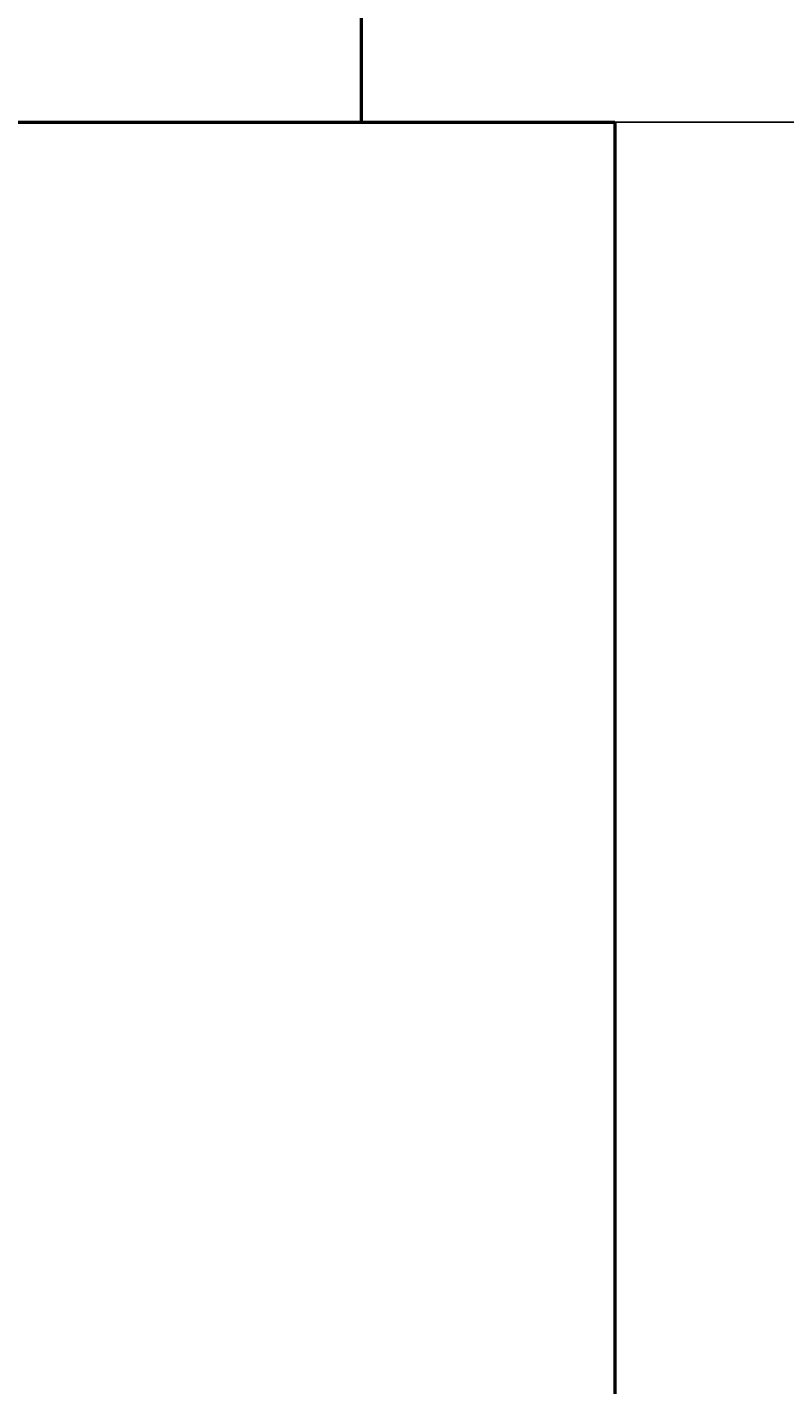
# Model space of a CAD drawing. Units: inches. Extents: x -173 to 545, y -746 to 104.
# Tile 16 of 32: x 278 to 314, y -528 to -463. Entities that reach past the tile are written whole.
import ezdxf

# ---------------------------------------------------------------- set-up
doc = ezdxf.new("R2010")
doc.units = ezdxf.units.IN
doc.header["$MEASUREMENT"] = 0
doc.layers.add('A-ANNO-DIMS', color=2, linetype='Continuous', lineweight=18)
doc.layers.add('A-WALL', color=7, linetype='Continuous', lineweight=50)
doc.styles.get("Standard").update_dxf_attribs({"font": 'arial.ttf'})
doc.dimstyles.get("Standard").update_dxf_attribs({"dimtxt": 0.18, "dimasz": 0.18, "dimexe": 0.18, "dimexo": 0.0625, "dimgap": 0.09, "dimtad": 0, "dimtih": 1, "dimtoh": 1, "dimdec": 0, "dimzin": 0, "dimdsep": 46, "dimlunit": 3, "dimtxsty": 'Standard', "dimcen": 0.09, "dimadec": 0, "dimazin": 0, "dimtfac": 1, "dimtdec": 0, "dimtofl": 0, "dimtmove": 0, "dimatfit": 3, "dimfxl": 1, "dimtolj": 1, "dimtzin": 0, "dimarcsym": 0})

# ---------------------------------------------------------------- blocks, each defined once
blk = doc.blocks.new('*D82')
at = {"layer": 'A-ANNO-DIMS', "color": 0, "lineweight": -2, "transparency": 16777216}
for p, q in [((219.864, -467.862), (545.081, -467.862)), ((544.901, -468.042), (544.901, -509.68)), ((544.901, -551.682), (544.901, -510.044)), ((219.864, -551.862), (545.081, -551.862))]:
    blk.add_line(p, q, dxfattribs=at)
at = {"layer": 'A-ANNO-DIMS', "color": 0, "transparency": 16777216}
for points in [[(544.871, -468.042), (544.931, -468.042), (544.901, -467.862)], [(544.871, -551.682), (544.931, -551.682), (544.901, -551.862)]]:
    blk.add_solid(points, dxfattribs=at)
at = {"layer": 'Defpoints', "color": 0, "transparency": 16777216}
for p in [(219.801, -467.862), (219.801, -551.862), (544.901, -551.862)]:
    blk.add_point(p, dxfattribs=at)
at = {"layer": 'A-ANNO-DIMS', "color": 0, "transparency": 16777216, "insert": (544.901, -509.862), "char_height": 0.18, "attachment_point": 5}
blk.add_mtext('\\A1;7\'-0"', dxfattribs=at)

msp = doc.modelspace()

# ---------------------------------------------------------------- linework, layer by layer
at = {"layer": 'A-WALL'}
for p, q in [((294.301, -458.862), (294.301, -467.862)), ((219.801, -467.862), (306.301, -467.862)), ((306.301, -467.862), (306.301, -551.862))]:
    msp.add_line(p, q, dxfattribs=at)

# ---------------------------------------------------------------- dimensions: what is measured, and where the dimension line sits
at = {"layer": 'A-ANNO-DIMS'}
dim = msp.add_linear_dim(base=(544.901, -551.862), p1=(219.801, -467.862), p2=(219.801, -551.862), angle=90, dimstyle='Standard', override={"dimdec": 1, "dimlfac": 1, "dimrnd": 0, "dimzin": 1, "dimdsep": 46, "dimlunit": 4, "dimfrac": 2}, dxfattribs=at)
dim.commit()
dim.dimension.update_dxf_attribs({"geometry": '*D82', "text_midpoint": (544.901, -509.862)})

doc.saveas('drawing.dxf')
